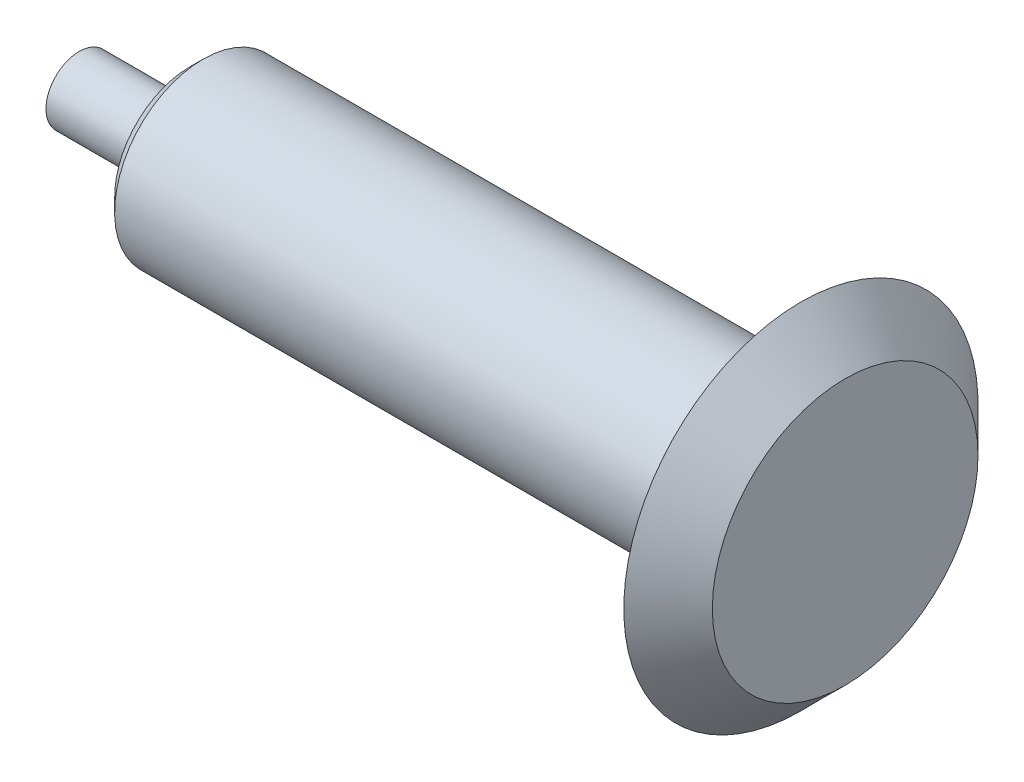
ISO-10303-21;
HEADER;
FILE_DESCRIPTION(('STEP AP214'),'2;1');
FILE_NAME('part.step','',(''),(''),'','','');
FILE_SCHEMA(('AUTOMOTIVE_DESIGN { 1 0 10303 214 1 1 1 1 }'));
ENDSEC;
DATA;
#1=APPLICATION_CONTEXT('core data for automotive mechanical design processes');
#2=APPLICATION_PROTOCOL_DEFINITION('international standard','automotive_design',2000,#1);
#3=PRODUCT_CONTEXT('',#1,'mechanical');
#4=PRODUCT('Part','Part','',(#3));
#5=PRODUCT_RELATED_PRODUCT_CATEGORY('part','',(#4));
#6=PRODUCT_DEFINITION_FORMATION('','',#4);
#7=PRODUCT_DEFINITION_CONTEXT('part definition',#1,'design');
#8=PRODUCT_DEFINITION('design','',#6,#7);
#9=PRODUCT_DEFINITION_SHAPE('','',#8);
#10=(LENGTH_UNIT() NAMED_UNIT(*) SI_UNIT(.MILLI.,.METRE.));
#11=(NAMED_UNIT(*) PLANE_ANGLE_UNIT() SI_UNIT($,.RADIAN.));
#12=(NAMED_UNIT(*) SI_UNIT($,.STERADIAN.) SOLID_ANGLE_UNIT());
#13=UNCERTAINTY_MEASURE_WITH_UNIT(LENGTH_MEASURE(1.E-05),#10,'distance_accuracy_value','');
#14=(GEOMETRIC_REPRESENTATION_CONTEXT(3) GLOBAL_UNCERTAINTY_ASSIGNED_CONTEXT((#13)) GLOBAL_UNIT_ASSIGNED_CONTEXT((#10,
#11,#12)) REPRESENTATION_CONTEXT('',''));
#15=CARTESIAN_POINT('',(0.,0.,0.));
#16=DIRECTION('',(0.,0.,1.));
#17=DIRECTION('',(1.,0.,0.));
#18=AXIS2_PLACEMENT_3D('',#15,#16,#17);
#19=CARTESIAN_POINT('',(145.,0.,0.));
#20=DIRECTION('',(-1.,0.,0.));
#21=DIRECTION('',(0.,-1.,0.));
#22=AXIS2_PLACEMENT_3D('',#19,#20,#21);
#23=PLANE('',#22);
#24=CARTESIAN_POINT('',(145.,0.,0.));
#25=DIRECTION('',(1.,0.,0.));
#26=DIRECTION('',(0.,1.,0.));
#27=AXIS2_PLACEMENT_3D('',#24,#25,#26);
#28=CIRCLE('',#27,30.0000000000003);
#29=CARTESIAN_POINT('',(145.,30.0000000000003,0.));
#30=VERTEX_POINT('',#29);
#31=EDGE_CURVE('E10',#30,#30,#28,.T.);
#32=ORIENTED_EDGE('',*,*,#31,.T.);
#33=EDGE_LOOP('',(#32));
#34=FACE_BOUND('',#33,.T.);
#35=ADVANCED_FACE('F39',(#34),#23,.F.);
#36=CARTESIAN_POINT('',(135.,0.,0.));
#37=DIRECTION('',(-1.,0.,0.));
#38=DIRECTION('',(0.,-1.,0.));
#39=AXIS2_PLACEMENT_3D('',#36,#37,#38);
#40=CONICAL_SURFACE('',#39,40.,0.785398163397432);
#41=ORIENTED_EDGE('',*,*,#31,.F.);
#42=EDGE_LOOP('',(#41));
#43=FACE_BOUND('',#42,.T.);
#44=CARTESIAN_POINT('',(135.,0.,0.));
#45=DIRECTION('',(1.,0.,0.));
#46=DIRECTION('',(0.,1.,0.));
#47=AXIS2_PLACEMENT_3D('',#44,#45,#46);
#48=CIRCLE('',#47,40.);
#49=CARTESIAN_POINT('',(135.,40.,0.));
#50=VERTEX_POINT('',#49);
#51=EDGE_CURVE('E44',#50,#50,#48,.T.);
#52=ORIENTED_EDGE('',*,*,#51,.T.);
#53=EDGE_LOOP('',(#52));
#54=FACE_BOUND('',#53,.T.);
#55=ADVANCED_FACE('F84',(#43,#54),#40,.T.);
#56=CARTESIAN_POINT('',(135.,0.,0.));
#57=DIRECTION('',(1.,0.,0.));
#58=DIRECTION('',(0.,1.,0.));
#59=AXIS2_PLACEMENT_3D('',#56,#57,#58);
#60=PLANE('',#59);
#61=ORIENTED_EDGE('',*,*,#51,.F.);
#62=EDGE_LOOP('',(#61));
#63=FACE_BOUND('',#62,.T.);
#64=CARTESIAN_POINT('',(135.,0.,0.));
#65=DIRECTION('',(1.,0.,0.));
#66=DIRECTION('',(0.,1.,0.));
#67=AXIS2_PLACEMENT_3D('',#64,#65,#66);
#68=CIRCLE('',#67,30.);
#69=CARTESIAN_POINT('',(135.,30.,0.));
#70=VERTEX_POINT('',#69);
#71=EDGE_CURVE('E47',#70,#70,#68,.T.);
#72=ORIENTED_EDGE('',*,*,#71,.T.);
#73=EDGE_LOOP('',(#72));
#74=FACE_BOUND('',#73,.T.);
#75=ADVANCED_FACE('F87',(#63,#74),#60,.F.);
#76=CARTESIAN_POINT('',(125.,0.,0.));
#77=DIRECTION('',(1.,0.,0.));
#78=DIRECTION('',(0.,1.,0.));
#79=AXIS2_PLACEMENT_3D('',#76,#77,#78);
#80=CONICAL_SURFACE('',#79,20.,0.785398163397449);
#81=ORIENTED_EDGE('',*,*,#71,.F.);
#82=EDGE_LOOP('',(#81));
#83=FACE_BOUND('',#82,.T.);
#84=CARTESIAN_POINT('',(125.,0.,0.));
#85=DIRECTION('',(1.,0.,0.));
#86=DIRECTION('',(0.,1.,0.));
#87=AXIS2_PLACEMENT_3D('',#84,#85,#86);
#88=CIRCLE('',#87,20.);
#89=CARTESIAN_POINT('',(125.,20.,0.));
#90=VERTEX_POINT('',#89);
#91=EDGE_CURVE('E52',#90,#90,#88,.T.);
#92=ORIENTED_EDGE('',*,*,#91,.T.);
#93=EDGE_LOOP('',(#92));
#94=FACE_BOUND('',#93,.T.);
#95=ADVANCED_FACE('F95',(#83,#94),#80,.T.);
#96=CARTESIAN_POINT('',(213.258902512884,0.,0.));
#97=DIRECTION('',(1.,0.,0.));
#98=DIRECTION('',(0.,1.,0.));
#99=AXIS2_PLACEMENT_3D('',#96,#97,#98);
#100=CYLINDRICAL_SURFACE('',#99,20.);
#101=ORIENTED_EDGE('',*,*,#91,.F.);
#102=EDGE_LOOP('',(#101));
#103=FACE_BOUND('',#102,.T.);
#104=CARTESIAN_POINT('',(0.,0.,0.));
#105=DIRECTION('',(1.,0.,0.));
#106=DIRECTION('',(0.,1.,0.));
#107=AXIS2_PLACEMENT_3D('',#104,#105,#106);
#108=CIRCLE('',#107,20.);
#109=CARTESIAN_POINT('',(0.,20.,0.));
#110=VERTEX_POINT('',#109);
#111=EDGE_CURVE('E59',#110,#110,#108,.T.);
#112=ORIENTED_EDGE('',*,*,#111,.T.);
#113=EDGE_LOOP('',(#112));
#114=FACE_BOUND('',#113,.T.);
#115=ADVANCED_FACE('F98',(#103,#114),#100,.T.);
#116=CARTESIAN_POINT('',(0.,0.,0.));
#117=DIRECTION('',(1.,0.,0.));
#118=DIRECTION('',(0.,1.,0.));
#119=AXIS2_PLACEMENT_3D('',#116,#117,#118);
#120=CONICAL_SURFACE('',#119,20.,0.785398163397456);
#121=CARTESIAN_POINT('',(-3.,0.,0.));
#122=DIRECTION('',(1.,0.,0.));
#123=DIRECTION('',(0.,1.,0.));
#124=AXIS2_PLACEMENT_3D('',#121,#122,#123);
#125=CIRCLE('',#124,17.);
#126=CARTESIAN_POINT('',(-3.,17.,0.));
#127=VERTEX_POINT('',#126);
#128=EDGE_CURVE('E62',#127,#127,#125,.T.);
#129=ORIENTED_EDGE('',*,*,#128,.T.);
#130=EDGE_LOOP('',(#129));
#131=FACE_BOUND('',#130,.T.);
#132=ORIENTED_EDGE('',*,*,#111,.F.);
#133=EDGE_LOOP('',(#132));
#134=FACE_BOUND('',#133,.T.);
#135=ADVANCED_FACE('F105',(#131,#134),#120,.T.);
#136=CARTESIAN_POINT('',(-3.,0.,0.));
#137=DIRECTION('',(1.,0.,0.));
#138=DIRECTION('',(0.,1.,0.));
#139=AXIS2_PLACEMENT_3D('',#136,#137,#138);
#140=PLANE('',#139);
#141=ORIENTED_EDGE('',*,*,#128,.F.);
#142=EDGE_LOOP('',(#141));
#143=FACE_BOUND('',#142,.T.);
#144=CARTESIAN_POINT('',(-3.,0.,0.));
#145=DIRECTION('',(1.,0.,0.));
#146=DIRECTION('',(0.,1.,0.));
#147=AXIS2_PLACEMENT_3D('',#144,#145,#146);
#148=CIRCLE('',#147,7.5);
#149=CARTESIAN_POINT('',(-3.,7.5,0.));
#150=VERTEX_POINT('',#149);
#151=EDGE_CURVE('E61',#150,#150,#148,.T.);
#152=ORIENTED_EDGE('',*,*,#151,.T.);
#153=EDGE_LOOP('',(#152));
#154=FACE_BOUND('',#153,.T.);
#155=ADVANCED_FACE('F78',(#143,#154),#140,.F.);
#156=CARTESIAN_POINT('',(213.258902512884,0.,0.));
#157=DIRECTION('',(1.,0.,0.));
#158=DIRECTION('',(0.,1.,0.));
#159=AXIS2_PLACEMENT_3D('',#156,#157,#158);
#160=CYLINDRICAL_SURFACE('',#159,7.5);
#161=CARTESIAN_POINT('',(-28.,0.,0.));
#162=DIRECTION('',(1.,0.,0.));
#163=DIRECTION('',(0.,1.,0.));
#164=AXIS2_PLACEMENT_3D('',#161,#162,#163);
#165=CIRCLE('',#164,7.5);
#166=CARTESIAN_POINT('',(-28.,7.5,0.));
#167=VERTEX_POINT('',#166);
#168=EDGE_CURVE('E67',#167,#167,#165,.T.);
#169=ORIENTED_EDGE('',*,*,#168,.T.);
#170=EDGE_LOOP('',(#169));
#171=FACE_BOUND('',#170,.T.);
#172=ORIENTED_EDGE('',*,*,#151,.F.);
#173=EDGE_LOOP('',(#172));
#174=FACE_BOUND('',#173,.T.);
#175=ADVANCED_FACE('F72',(#171,#174),#160,.T.);
#176=CARTESIAN_POINT('',(-28.,0.,0.));
#177=DIRECTION('',(-1.,0.,0.));
#178=DIRECTION('',(0.,-1.,0.));
#179=AXIS2_PLACEMENT_3D('',#176,#177,#178);
#180=PLANE('',#179);
#181=ORIENTED_EDGE('',*,*,#168,.F.);
#182=EDGE_LOOP('',(#181));
#183=FACE_BOUND('',#182,.T.);
#184=ADVANCED_FACE('F74',(#183),#180,.T.);
#185=CLOSED_SHELL('',(#35,#55,#75,#95,#115,#135,#155,#175,#184));
#186=MANIFOLD_SOLID_BREP('B2',#185);
#187=ADVANCED_BREP_SHAPE_REPRESENTATION('',(#18,#186),#14);
#188=SHAPE_DEFINITION_REPRESENTATION(#9,#187);
ENDSEC;
END-ISO-10303-21;
